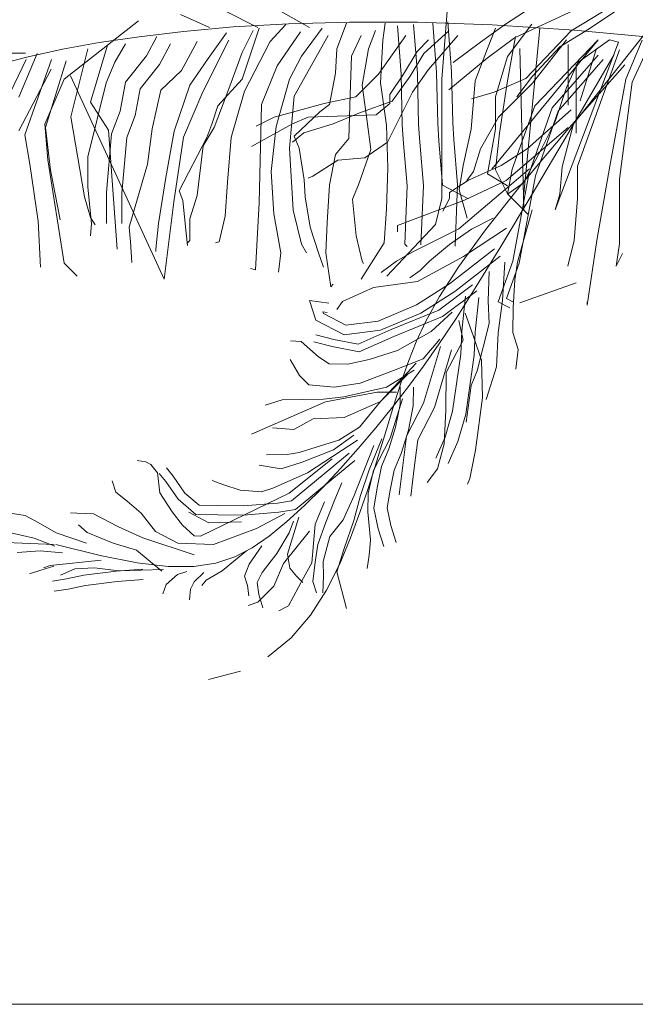
# Model space of a CAD drawing. Units: millimetres. Extents: x 595116 to 630915, y 909473 to 920225.
# Tile 96 of 134: x 629798.32 to 629805.27, y 919160.92 to 919172.02. Entities that reach past the tile are written whole.
import ezdxf

# ---------------------------------------------------------------- set-up
doc = ezdxf.new("R2010")
doc.units = ezdxf.units.MM
doc.layers.add('L-PLNT', color=85, linetype='Continuous', lineweight=13)

# ---------------------------------------------------------------- blocks, each defined once
blk = doc.blocks.new('A$C4FB75ABC')
for p, q in [((2.1065, 2.3741), (2.087, 2.1315)), ((2.2781, 2.2963), (2.353, 2.344)), ((2.3054, 2.2555), (2.4825, 2.3372)), ((2.5983, 2.3508), (2.4757, 2.2759)), ((2.6119, 2.3372), (2.5302, 2.2827)), ((1.3881, 2.2867), (1.3008, 2.3255)), ((1.5337, 2.2867), (1.4367, 2.3352)), ((1.6891, 2.2867), (1.6017, 2.3352)), ((1.1746, 2.3061), (0.9513, 2.1315)), ((1.4598, 2.2878), (1.3106, 2.2744)), ((1.6258, 2.2976), (1.4598, 2.2878)), ((1.5376, 2.2844), (1.4866, 2.1313)), ((1.6179, 2.2954), (1.5705, 2.2443)), ((1.8099, 2.3026), (1.6258, 2.2976)), ((1.7274, 2.2844), (1.6654, 2.2006)), ((1.8004, 2.299), (1.7712, 2.2224)), ((2.0136, 2.3019), (1.8099, 2.3026)), ((1.9171, 2.299), (1.9098, 2.248)), ((1.9536, 2.2917), (1.9646, 2.1459)), ((2.0023, 2.2954), (2.0134, 2.1483)), ((2.2382, 2.2942), (2.0136, 2.3019)), ((2.0597, 2.2997), (2.0708, 2.1511)), ((2.1047, 2.3031), (2.1159, 2.1533)), ((2.2032, 2.2419), (2.2781, 2.2963)), ((2.2482, 2.2839), (2.2239, 2.2232)), ((2.4852, 2.2785), (2.2382, 2.2942)), ((2.3575, 2.296), (2.2846, 2.199)), ((2.3818, 2.2839), (2.3332, 1.7863)), ((2.5302, 2.2827), (2.4416, 2.2282)), ((2.7559, 2.2536), (2.4852, 2.2785)), ((1.1767, 2.2586), (1.0564, 2.241)), ((1.3106, 2.2744), (1.1767, 2.2586)), ((1.23, 2.2589), (1.1992, 2.2008)), ((1.4391, 2.2699), (1.3844, 2.1933)), ((1.5194, 2.2771), (1.4866, 2.2115)), ((1.6617, 2.2735), (1.5924, 2.1714)), ((1.7456, 2.2626), (1.6435, 2.0802)), ((1.8442, 2.2626), (1.815, 2.2006)), ((1.8879, 2.2771), (1.8661, 2.2224)), ((1.9783, 2.2623), (1.8966, 2.1465)), ((2.0124, 2.2146), (2.0465, 2.2487)), ((2.1078, 2.2759), (2.0328, 2.2078)), ((2.135, 2.2623), (2.0465, 2.1602)), ((2.2236, 2.1942), (2.3054, 2.2555)), ((2.5574, 2.2487), (2.2372, 1.8605)), ((2.3089, 2.2596), (2.2846, 2.1261)), ((2.4757, 2.2759), (2.3394, 2.1329)), ((2.462, 2.2487), (2.3599, 2.1193)), ((2.3667, 2.0512), (2.5574, 2.2487)), ((2.6937, 2.2623), (2.4825, 1.9967)), ((2.5915, 2.2487), (2.4961, 2.1806)), ((2.6187, 2.2419), (2.5915, 2.2487)), ((0.9464, 2.2213), (0.8429, 2.1986)), ((1.0564, 2.241), (0.9464, 2.2213)), ((1.0231, 2.2224), (0.972, 2.0182)), ((1.0815, 2.2334), (1.0304, 2.062)), ((1.1363, 2.237), (1.1034, 2.1823)), ((1.2713, 2.237), (1.2384, 2.175)), ((1.3515, 2.2443), (1.3041, 2.1568)), ((1.4464, 2.2479), (1.3687, 2.0927)), ((1.5705, 2.2443), (1.4939, 2.0948)), ((1.7712, 2.2224), (1.7675, 2.1495)), ((1.8661, 2.2224), (1.8478, 2.113)), ((1.9098, 2.248), (1.9025, 2.1203)), ((2.1214, 2.1806), (2.2032, 2.2419)), ((2.2239, 2.2232), (2.1875, 2.1261)), ((2.3211, 2.2232), (2.3332, 1.7378)), ((2.4416, 2.2282), (2.3599, 2.1397)), ((2.428, 1.738), (2.6187, 2.2419)), ((2.4668, 2.2354), (2.4668, 2.0533)), ((2.6209, 2.2188), (2.4948, 1.8695)), ((2.5518, 2.2232), (2.5032, 2.0655)), ((2.6889, 2.2479), (2.6404, 2.1315)), ((2.7083, 2.2285), (2.6598, 2.1218)), ((0.837, 2.1896), (0.7276, 1.9635)), ((0.8429, 2.1986), (0.7422, 2.1723)), ((0.8348, 2.2091), (0.7572, 2.2091)), ((0.8699, 2.2079), (0.8151, 2.0766)), ((0.9137, 2.1896), (0.8334, 1.9635)), ((1.1992, 2.2008), (1.1362, 2.1221)), ((1.3844, 2.1933), (1.3297, 2.113)), ((1.4866, 2.2115), (1.4464, 2.1021)), ((1.6654, 2.2006), (1.6289, 2.1313)), ((1.815, 2.2006), (1.8113, 2.0838)), ((1.9715, 2.1465), (2.0124, 2.2146)), ((2.0328, 2.2078), (1.992, 2.1397)), ((2.1078, 2.0989), (2.2236, 2.1942)), ((2.2846, 2.199), (2.2482, 2.0776)), ((2.5572, 2.203), (2.4187, 2.0449)), ((2.5724, 2.1897), (2.4365, 2.0345)), ((2.6056, 2.2048), (2.4676, 1.9701)), ((0.9125, 2.1606), (0.8154, 1.9763)), ((0.9575, 2.186), (0.8954, 1.9854)), ((1.1034, 2.1823), (1.0779, 2.1203)), ((1.2384, 2.175), (1.18, 2.1021)), ((1.5924, 2.1714), (1.5449, 2.0547)), ((2.0465, 2.1602), (1.9988, 2.0921)), ((2.4961, 2.1806), (2.462, 2.1057)), ((2.6368, 2.1742), (2.4628, 1.9766)), ((2.4911, 2.1747), (2.4911, 1.9684)), ((0.9513, 2.1315), (0.8931, 1.9957)), ((1.2522, 1.53), (0.9707, 2.1412)), ((1.3041, 2.1568), (1.2421, 2.0984)), ((1.4866, 2.1313), (1.4136, 2.051)), ((1.6289, 2.1313), (1.5887, 1.989)), ((1.7675, 2.1495), (1.7493, 2.0547)), ((1.8966, 2.1465), (1.8285, 2.0784)), ((1.9306, 2.0852), (1.9715, 2.1465)), ((1.992, 2.1397), (1.9375, 2.0648)), ((1.9646, 2.1459), (1.9682, 1.9927)), ((2.0134, 2.1483), (2.017, 1.9949)), ((2.0708, 2.1511), (2.0745, 1.9975)), ((2.087, 2.1315), (2.087, 1.7725)), ((2.1159, 2.1533), (2.1196, 1.9995)), ((2.3394, 2.1329), (2.244, 2.0921)), ((2.3599, 2.1397), (2.3122, 2.0784)), ((2.6404, 2.1315), (2.5918, 1.8695)), ((1.0779, 2.1203), (1.0231, 1.8978)), ((1.1362, 2.1221), (1.1203, 2.0346)), ((1.18, 2.1021), (1.1654, 2.0218)), ((1.3297, 2.113), (1.2822, 1.9744)), ((1.4464, 2.1021), (1.4026, 1.9854)), ((1.8478, 2.113), (1.8624, 2.0036)), ((1.9025, 2.1203), (1.9208, 1.9927)), ((2.1875, 2.1261), (2.1754, 1.9805)), ((2.3599, 2.1193), (2.2577, 2.0172)), ((2.2846, 2.1261), (2.2604, 1.9684)), ((2.462, 2.1057), (2.428, 2.0035)), ((2.6598, 2.1218), (2.6209, 1.8307)), ((1.2421, 2.0984), (1.2165, 1.9817)), ((1.3687, 2.0927), (1.3105, 1.9569)), ((1.4939, 2.0948), (1.4537, 1.9562)), ((1.6435, 2.0802), (1.6289, 1.9234)), ((1.8285, 2.0784), (1.7331, 2.058)), ((1.8113, 2.0838), (1.8077, 1.9526)), ((1.9988, 2.0921), (1.9238, 1.9422)), ((1.9306, 2.058), (1.9306, 2.0852)), ((2.244, 2.0921), (2.1759, 2.0716)), ((2.2482, 2.0776), (2.2482, 1.9805)), ((1.0304, 2.062), (1.0852, 1.9781)), ((1.4136, 2.051), (1.3953, 1.9963)), ((1.5449, 2.0547), (1.5376, 1.7593)), ((1.7331, 2.058), (1.5832, 2.0172)), ((1.7493, 2.0547), (1.7201, 2.0328)), ((1.9375, 2.0648), (1.8421, 2.0308)), ((1.8898, 2.024), (1.9306, 2.058)), ((2.2985, 1.8605), (2.3667, 2.0512)), ((2.4187, 2.0449), (2.3489, 1.8456)), ((0.972, 2.0182), (1.0122, 1.7775)), ((1.1203, 2.0346), (1.0939, 1.9669)), ((1.1654, 2.0218), (1.1399, 1.9562)), ((1.5832, 2.0172), (1.5287, 1.9899)), ((1.6377, 1.9967), (1.6854, 2.0172)), ((1.7201, 2.0328), (1.6435, 1.9598)), ((1.6854, 2.0172), (1.8898, 2.024)), ((1.8421, 2.0308), (1.7603, 1.9967)), ((2.2577, 2.0172), (2.2032, 1.9218)), ((2.4756, 2.0387), (2.3438, 1.9217)), ((2.4365, 2.0345), (2.3686, 1.8404)), ((0.8931, 1.9957), (0.9028, 1.8889)), ((0.8954, 1.9854), (0.91, 1.8577)), ((1.4026, 1.9854), (1.3698, 1.9307)), ((1.3953, 1.9963), (1.3807, 1.9562)), ((1.5151, 1.9286), (1.6377, 1.9967)), ((1.5887, 1.989), (1.5741, 1.8541)), ((1.7603, 1.9967), (1.6718, 1.9695)), ((1.8624, 2.0036), (1.8734, 1.9197)), ((1.9208, 1.9927), (1.9244, 1.865)), ((1.9682, 1.9927), (1.9719, 1.938)), ((2.017, 1.9949), (2.0206, 1.9417)), ((2.0745, 1.9975), (2.0779, 1.946)), ((2.1196, 1.9995), (2.1229, 1.9495)), ((2.4673, 1.986), (2.2802, 1.8264)), ((2.428, 2.0035), (2.3871, 1.9218)), ((2.4825, 1.9967), (2.4484, 1.8673)), ((0.8334, 1.9635), (0.848, 1.876)), ((1.0939, 1.9669), (1.0786, 1.7905)), ((1.0852, 1.9781), (1.1107, 1.6207)), ((1.1399, 1.9562), (1.1253, 1.7884)), ((1.2165, 1.9817), (1.2019, 1.876)), ((1.2822, 1.9744), (1.2567, 1.8358)), ((1.3105, 1.9569), (1.2814, 1.7628)), ((1.3807, 1.9562), (1.2968, 1.7957)), ((1.4537, 1.9562), (1.4428, 1.8213)), ((1.6718, 1.9695), (1.6377, 1.9422)), ((1.6435, 1.9598), (1.6581, 1.9234)), ((1.8077, 1.9526), (1.7675, 1.9051)), ((2.1754, 1.9805), (2.1511, 1.8713)), ((2.2482, 1.9805), (2.2239, 1.847)), ((2.2604, 1.9684), (2.2482, 1.8591)), ((2.4628, 1.9766), (2.3249, 1.8127)), ((2.4676, 1.9701), (2.3552, 1.7802)), ((1.3698, 1.9307), (1.3515, 1.7811)), ((1.6289, 1.9234), (1.6398, 1.7374)), ((1.6581, 1.9234), (1.6727, 1.8285)), ((1.9238, 1.9422), (1.8557, 1.8946)), ((1.9719, 1.938), (1.9828, 1.8103)), ((2.0206, 1.9417), (2.0317, 1.8114)), ((2.0779, 1.946), (2.0893, 1.8127)), ((2.1229, 1.9495), (2.1345, 1.8136)), ((1.0231, 1.8978), (1.0231, 1.8067)), ((1.7675, 1.9051), (1.7493, 1.814)), ((1.8557, 1.8946), (1.7739, 1.8878)), ((1.8734, 1.9197), (1.8369, 1.814)), ((2.2032, 1.9218), (2.1827, 1.8537)), ((2.3438, 1.9217), (2.2657, 1.8718)), ((2.3871, 1.9218), (2.3326, 1.8197)), ((0.848, 1.876), (0.8735, 1.7045)), ((0.9028, 1.8889), (0.9513, 1.5785)), ((1.2019, 1.876), (1.1472, 1.6863)), ((1.7739, 1.8878), (1.699, 1.8401)), ((1.9244, 1.865), (1.9208, 1.741)), ((2.1511, 1.8713), (2.1389, 1.7985)), ((2.2657, 1.8718), (2.167, 1.8279)), ((2.4484, 1.8673), (2.4416, 1.7856)), ((2.4948, 1.8695), (2.4948, 1.7725)), ((2.5918, 1.8695), (2.553, 1.6464)), ((0.91, 1.8577), (0.9392, 1.7082)), ((1.2567, 1.8358), (1.2348, 1.6973)), ((1.5741, 1.8541), (1.5814, 1.7264)), ((1.699, 1.8401), (1.6854, 1.8333)), ((2.3505, 1.8613), (2.1386, 1.6813)), ((2.1827, 1.8537), (2.1623, 1.8265)), ((2.2239, 1.847), (2.2846, 1.8106)), ((2.2482, 1.8591), (2.2846, 1.7863)), ((2.2849, 1.7856), (2.2985, 1.8605)), ((2.3489, 1.8456), (2.3004, 1.5838)), ((2.3686, 1.8404), (2.32, 1.5785)), ((1.0231, 1.8067), (1.0341, 1.6973)), ((1.4428, 1.8213), (1.4355, 1.7191)), ((1.6727, 1.8285), (1.6763, 1.7775)), ((1.7493, 1.814), (1.742, 1.7009)), ((1.8369, 1.814), (1.8186, 1.7702)), ((1.9828, 1.8103), (1.9755, 1.6352)), ((2.0317, 1.8114), (2.0243, 1.6332)), ((2.0893, 1.8127), (2.1647, 1.7725)), ((2.167, 1.8279), (2.1099, 1.791)), ((2.1345, 1.8136), (2.1268, 1.6289)), ((2.2802, 1.8264), (2.1549, 1.7678)), ((2.3249, 1.8127), (2.2184, 1.678)), ((2.3326, 1.8197), (2.2849, 1.7856)), ((2.6209, 1.8307), (2.6209, 1.6367)), ((1.0122, 1.7775), (1.0304, 1.7155)), ((1.0786, 1.7905), (1.0786, 1.6973)), ((1.1253, 1.7884), (1.1253, 1.7665)), ((1.2968, 1.7957), (1.3078, 1.7665)), ((1.3515, 1.7811), (1.3297, 1.7118)), ((1.6763, 1.7775), (1.6909, 1.6863)), ((2.1099, 1.791), (2.1096, 1.7722)), ((2.1389, 1.7985), (2.1632, 1.7135)), ((2.3552, 1.7802), (2.2641, 1.6283)), ((2.2846, 1.7863), (2.3453, 1.7256)), ((2.4416, 1.7856), (2.428, 1.738)), ((1.1253, 1.7665), (1.1253, 1.7301)), ((1.2814, 1.7628), (1.2522, 1.53)), ((1.3078, 1.7665), (1.3187, 1.6681)), ((1.5376, 1.7593), (1.5267, 1.5587)), ((1.8186, 1.7702), (1.8296, 1.6608)), ((2.1549, 1.7678), (1.9538, 1.6913)), ((2.087, 1.7725), (2.0676, 1.6949)), ((2.1096, 1.7722), (2.0903, 1.7347)), ((2.4948, 1.7725), (2.485, 1.6464)), ((1.1253, 1.7301), (1.1253, 1.6973)), ((1.4355, 1.7191), (1.4172, 1.6425)), ((1.5814, 1.7264), (1.6033, 1.6097)), ((1.6398, 1.7374), (1.6654, 1.6352)), ((1.9208, 1.741), (1.9135, 1.6389)), ((2.3582, 1.7386), (2.3145, 1.5808)), ((0.8735, 1.7045), (0.8808, 1.566)), ((1.0304, 1.7155), (1.045, 1.6936)), ((1.0341, 1.6973), (1.0304, 1.6608)), ((1.1472, 1.6863), (1.1509, 1.6425)), ((1.2348, 1.6973), (1.2275, 1.6207)), ((1.3297, 1.7118), (1.3297, 1.6462)), ((1.6909, 1.6863), (1.7164, 1.6097)), ((1.742, 1.7009), (1.7383, 1.6097)), ((2.0676, 1.6949), (1.922, 1.5397)), ((1.9538, 1.6913), (1.9536, 1.6725)), ((2.2409, 1.7138), (2.1763, 1.6807)), ((1.3187, 1.6681), (1.3224, 1.6316)), ((1.8296, 1.6608), (1.8478, 1.5842)), ((2.1386, 1.6813), (1.998, 1.6115)), ((2.1763, 1.6807), (2.1096, 1.6345)), ((2.2184, 1.678), (2.1385, 1.568)), ((2.2819, 1.6831), (2.1525, 1.5981)), ((1.1509, 1.6425), (1.1545, 1.5805)), ((1.3297, 1.6462), (1.3224, 1.6389)), ((1.4172, 1.6425), (1.4063, 1.6389)), ((1.6654, 1.6352), (1.68, 1.6097)), ((1.9135, 1.6389), (1.8444, 1.53)), ((1.9755, 1.6352), (1.9828, 1.628)), ((2.1096, 1.6345), (2.0504, 1.5844)), ((2.2641, 1.6283), (2.1904, 1.5079)), ((2.485, 1.6464), (2.4656, 1.5688)), ((2.553, 1.6464), (2.5239, 1.4523)), ((2.6209, 1.6367), (2.6112, 1.5688)), ((1.2275, 1.6207), (1.2275, 1.6134)), ((1.6033, 1.6097), (1.596, 1.5514)), ((1.7164, 1.6097), (1.731, 1.566)), ((1.7383, 1.6097), (1.7529, 1.5076)), ((1.998, 1.6115), (1.9504, 1.5839)), ((2.1525, 1.5981), (2.0137, 1.5227)), ((2.2452, 1.6213), (2.1098, 1.5157)), ((2.2623, 1.5995), (2.1258, 1.493)), ((2.6112, 1.5688), (2.6307, 1.6076)), ((0.9513, 1.5785), (0.9901, 1.5397)), ((1.8478, 1.5842), (1.8515, 1.5769)), ((1.9504, 1.5839), (1.9047, 1.5506)), ((2.0504, 1.5844), (2.0217, 1.5565)), ((2.1385, 1.568), (2.0803, 1.4783)), ((2.3004, 1.5838), (2.256, 1.4617)), ((2.2767, 1.5813), (2.2695, 1.4664)), ((2.32, 1.5785), (2.2812, 1.4717)), ((2.3145, 1.5808), (2.3062, 1.5281)), ((1.5267, 1.5587), (1.5121, 1.5623)), ((2.0217, 1.5565), (1.9912, 1.5343)), ((2.2292, 1.5537), (2.2261, 1.4651)), ((1.7529, 1.5076), (1.7602, 1.5149)), ((2.0137, 1.5227), (1.8814, 1.5056)), ((2.1098, 1.5157), (2.0109, 1.453)), ((2.1796, 1.5129), (2.0785, 1.437)), ((2.3062, 1.5281), (2.3013, 1.4452)), ((2.4911, 1.5193), (2.3211, 1.4586)), ((1.8814, 1.5056), (1.7884, 1.4636)), ((2.1258, 1.493), (2.0238, 1.4284)), ((2.1927, 1.4954), (2.0894, 1.4177)), ((2.1904, 1.5079), (2.1298, 1.4122)), ((2.1578, 1.4791), (2.1468, 1.3743)), ((1.7084, 1.4073), (1.6895, 1.4666)), ((1.6895, 1.4666), (1.747, 1.4576)), ((1.7884, 1.4636), (1.7711, 1.4393)), ((2.0109, 1.453), (1.8951, 1.4036)), ((2.0803, 1.4783), (2.039, 1.4043)), ((2.1979, 1.4749), (2.187, 1.3714)), ((2.2261, 1.4651), (2.2289, 1.3972)), ((2.256, 1.4617), (2.2916, 1.4439)), ((2.2695, 1.4664), (2.2568, 1.3685)), ((2.2812, 1.4717), (2.3006, 1.462)), ((2.5239, 1.4523), (2.5239, 1.462)), ((1.7313, 1.4266), (1.7295, 1.4323)), ((1.7295, 1.4323), (1.7427, 1.4302)), ((1.7987, 1.3918), (1.7313, 1.4266)), ((2.0238, 1.4284), (1.9024, 1.3766)), ((2.0785, 1.437), (1.9344, 1.3786)), ((2.1181, 1.4308), (2.055, 1.3732)), ((2.1569, 1.4277), (2.1816, 1.3609)), ((2.3013, 1.4452), (2.3002, 1.3698)), ((1.7936, 1.3632), (1.7084, 1.4073)), ((1.8951, 1.4036), (1.7987, 1.3918)), ((2.0894, 1.4177), (1.9429, 1.3584)), ((2.039, 1.4043), (2.0098, 1.3416)), ((2.1298, 1.4122), (2.0784, 1.3347)), ((2.1385, 1.406), (2.1509, 1.3473)), ((2.2289, 1.3972), (2.1929, 1.2544)), ((1.7623, 1.3489), (1.7078, 1.3628)), ((1.9024, 1.3766), (1.7936, 1.3632)), ((1.9344, 1.3786), (1.8357, 1.3347)), ((2.055, 1.3732), (1.9542, 1.3161)), ((2.1468, 1.3743), (2.1439, 1.3053)), ((2.1816, 1.3609), (2.2062, 1.287)), ((2.187, 1.3714), (2.1842, 1.3016)), ((2.2568, 1.3685), (2.2516, 1.2668)), ((2.3002, 1.3698), (2.3165, 1.3187)), ((1.6641, 1.3427), (1.6321, 1.345)), ((1.7163, 1.2967), (1.6641, 1.3427)), ((1.7575, 1.3275), (1.7024, 1.3416)), ((1.8357, 1.3347), (1.7623, 1.3489)), ((1.9429, 1.3584), (1.8383, 1.3119)), ((2.0098, 1.3416), (1.9878, 1.2857)), ((2.0811, 1.3502), (2.0312, 1.2905)), ((2.0784, 1.3347), (2.0319, 1.2687)), ((2.1509, 1.3473), (2.1005, 1.25)), ((1.8383, 1.3119), (1.7575, 1.3275)), ((1.9542, 1.3161), (1.869, 1.289)), ((2.0829, 1.3276), (2.0324, 1.158)), ((2.1165, 1.3176), (2.065, 1.1449)), ((2.1439, 1.3053), (2.1195, 1.1332)), ((2.1842, 1.3016), (2.1591, 1.1247)), ((2.3165, 1.3187), (2.31, 1.2603)), ((1.6589, 1.2409), (1.6313, 1.2885)), ((1.7481, 1.2755), (1.7163, 1.2967)), ((1.8046, 1.2748), (1.7481, 1.2755)), ((1.869, 1.289), (1.8046, 1.2748)), ((2.0103, 1.2776), (1.903, 1.1622)), ((2.0312, 1.2905), (1.9421, 1.2559)), ((1.9878, 1.2857), (1.9691, 1.2327)), ((2.2062, 1.287), (2.2097, 1.1745)), ((1.9421, 1.2559), (1.8416, 1.2177)), ((1.9834, 1.244), (1.903, 1.1622)), ((2.0043, 1.257), (1.9206, 1.2053)), ((2.0319, 1.2687), (1.9864, 1.2075)), ((2.1005, 1.25), (2.0989, 1.1369)), ((2.1929, 1.2544), (2.1754, 1.2112)), ((2.2516, 1.2668), (2.22, 1.1691)), ((1.6868, 1.2123), (1.6589, 1.2409)), ((1.8416, 1.2177), (1.7641, 1.2056)), ((1.9691, 1.2327), (1.952, 1.1808)), ((1.7641, 1.2056), (1.6868, 1.2123)), ((1.7376, 1.1613), (1.8929, 1.1904)), ((1.9206, 1.2053), (1.792, 1.1769)), ((1.8929, 1.1904), (1.9511, 1.1904)), ((1.9864, 1.2075), (1.9386, 1.1458)), ((1.9621, 1.2066), (1.9614, 1.1536)), ((2.0017, 1.2061), (2.001, 1.1495)), ((2.1754, 1.2112), (2.1606, 1.1002)), ((1.5143, 1.0642), (1.7376, 1.1613)), ((1.607, 1.1681), (1.5558, 1.1518)), ((1.7315, 1.1702), (1.607, 1.1681)), ((1.792, 1.1769), (1.7315, 1.1702)), ((1.903, 1.1622), (1.793, 1.1147)), ((1.903, 1.1622), (1.8397, 1.0857)), ((1.9692, 1.1707), (1.9317, 1.0524)), ((1.952, 1.1808), (1.9358, 1.129)), ((1.9614, 1.1536), (1.9482, 1.0859)), ((2.0324, 1.158), (1.9806, 1.0581)), ((2.2097, 1.1745), (2.1886, 1.0162)), ((1.9386, 1.1458), (1.8882, 1.0835)), ((1.9358, 1.129), (1.9198, 1.076)), ((2.001, 1.1495), (1.9867, 1.0762)), ((2.065, 1.1449), (2.0146, 1.0475)), ((2.0989, 1.1369), (2.0937, 1.0351)), ((2.1195, 1.1332), (2.0972, 1.056)), ((2.1591, 1.1247), (2.1353, 1.0421)), ((1.7005, 1.1103), (1.6416, 1.079)), ((1.793, 1.1147), (1.7005, 1.1103)), ((1.6416, 1.079), (1.5775, 1.0837)), ((1.8397, 1.0857), (1.7769, 1.047)), ((1.8882, 1.0835), (1.8359, 1.0215)), ((1.9198, 1.076), (1.903, 1.0206)), ((1.9482, 1.0859), (1.9278, 1.0204)), ((1.9867, 1.0762), (1.965, 1.0067)), ((1.8335, 1.0462), (1.6831, 0.9483)), ((1.7769, 1.047), (1.7087, 1.0253)), ((1.8224, 1.0615), (1.7614, 1.017)), ((1.9071, 1.0509), (1.8681, 0.9571)), ((1.9317, 1.0524), (1.8813, 0.9551)), ((1.9806, 1.0581), (1.9586, 0.8825)), ((2.0146, 1.0475), (2.004, 0.9628)), ((2.0972, 1.056), (2.0692, 0.9929)), ((2.1353, 1.0421), (2.1061, 0.9765)), ((1.6576, 1.009), (1.6216, 1.0039)), ((1.8084, 1.007), (1.6348, 0.8642)), ((1.7087, 1.0253), (1.6576, 1.009)), ((1.7614, 1.017), (1.6666, 0.9806)), ((1.8359, 1.0215), (1.7823, 0.9612)), ((1.8823, 1.0305), (1.8549, 0.9592)), ((1.903, 1.0206), (1.8847, 0.9618)), ((1.9278, 1.0204), (1.9055, 0.9679)), ((1.965, 1.0067), (1.9435, 0.9561)), ((2.0937, 1.0351), (2.0738, 0.96)), ((2.1886, 1.0162), (2.171, 0.9318)), ((1.1969, 0.9814), (1.1705, 0.9855)), ((1.2119, 0.9737), (1.1969, 0.9814)), ((1.6216, 1.0039), (1.5594, 1.0028)), ((1.6666, 0.9806), (1.6041, 0.9607)), ((1.7573, 0.9907), (1.6276, 0.8869)), ((1.8259, 0.9857), (1.6466, 0.8382)), ((1.2323, 0.9489), (1.2119, 0.9737)), ((1.239, 0.8884), (1.2323, 0.9489)), ((1.2793, 0.9388), (1.2589, 0.9636)), ((1.6041, 0.9607), (1.5382, 0.9711)), ((1.6831, 0.9483), (1.5787, 0.9026)), ((1.7823, 0.9612), (1.7281, 0.9036)), ((1.8549, 0.9592), (1.8236, 0.8804)), ((1.8681, 0.9571), (1.8425, 0.8802)), ((1.8847, 0.9618), (1.8642, 0.8983)), ((1.8813, 0.9551), (1.8652, 0.8874)), ((1.9055, 0.9679), (1.8924, 0.9029)), ((1.9435, 0.9561), (1.9314, 0.8959)), ((2.004, 0.9628), (1.9934, 0.8781)), ((2.0738, 0.96), (2.043, 0.9189)), ((1.107, 0.8902), (1.0961, 0.9243)), ((1.2572, 0.9222), (1.2376, 0.9461)), ((1.2938, 0.8688), (1.2572, 0.9222)), ((1.3144, 0.8874), (1.2793, 0.9388)), ((1.4036, 0.922), (1.3961, 0.9259)), ((1.4317, 0.9122), (1.4036, 0.922)), ((1.7864, 0.9186), (1.765, 0.868)), ((2.171, 0.9318), (2.164, 0.9142)), ((1.1405, 0.8634), (1.107, 0.8902)), ((1.2759, 0.8314), (1.239, 0.8884)), ((1.3573, 0.851), (1.3144, 0.8874)), ((1.4805, 0.8964), (1.4317, 0.9122)), ((1.5446, 0.8918), (1.4805, 0.8964)), ((1.5787, 0.9026), (1.5446, 0.8918)), ((1.7281, 0.9036), (1.6739, 0.8498)), ((1.8642, 0.8983), (1.8405, 0.829)), ((1.8652, 0.8874), (1.8644, 0.8308)), ((1.8924, 0.9029), (1.8829, 0.8424)), ((1.9314, 0.8959), (1.9231, 0.8432)), ((1.1834, 0.827), (1.1405, 0.8634)), ((1.347, 0.8236), (1.2938, 0.8688)), ((1.6276, 0.8869), (1.3617, 0.7585)), ((1.6348, 0.8642), (1.5932, 0.8572)), ((1.7347, 0.8614), (1.7065, 0.7946)), ((1.765, 0.868), (1.7376, 0.7967)), ((1.8236, 0.8804), (1.7906, 0.8073)), ((1.8425, 0.8802), (1.8226, 0.805)), ((1.3074, 0.7913), (1.2759, 0.8314)), ((1.3863, 0.7981), (1.3265, 0.8298)), ((1.4139, 0.8502), (1.3573, 0.851)), ((1.4893, 0.8492), (1.4139, 0.8502)), ((1.5932, 0.8572), (1.4893, 0.8492)), ((1.5965, 0.8298), (1.4902, 0.8216)), ((1.6466, 0.8382), (1.5965, 0.8298)), ((1.6739, 0.8498), (1.6204, 0.8011)), ((1.8405, 0.829), (1.8129, 0.7535)), ((1.8644, 0.8308), (1.8727, 0.7459)), ((1.8829, 0.8424), (1.8952, 0.7804)), ((1.9231, 0.8432), (1.9337, 0.7903)), ((0.8346, 0.8198), (0.7888, 0.827)), ((0.8736, 0.7996), (0.8346, 0.8198)), ((0.9273, 0.7678), (0.8736, 0.7996)), ((0.9891, 0.8277), (0.9703, 0.828)), ((1.04, 0.8252), (0.9891, 0.8277)), ((1.1149, 0.7864), (1.04, 0.8252)), ((1.226, 0.7717), (1.1834, 0.827)), ((1.4135, 0.8227), (1.347, 0.8236)), ((1.4848, 0.8016), (1.3863, 0.7981)), ((1.4902, 0.8216), (1.4135, 0.8227)), ((1.6154, 0.8267), (1.5299, 0.7807)), ((1.6204, 0.8011), (1.5682, 0.7585)), ((1.6567, 0.8148), (1.6231, 0.704)), ((1.6415, 0.8037), (1.6278, 0.7681)), ((1.7906, 0.8073), (1.7502, 0.757)), ((1.8226, 0.805), (1.7931, 0.7206)), ((1.0204, 0.7689), (0.9943, 0.7918)), ((1.188, 0.7534), (1.1149, 0.7864)), ((1.2935, 0.7368), (1.226, 0.7717)), ((1.3428, 0.7588), (1.3074, 0.7913)), ((1.5299, 0.7807), (1.4009, 0.7335)), ((1.6891, 0.7732), (1.6114, 0.6762)), ((1.7065, 0.7946), (1.696, 0.6785)), ((1.7376, 0.7967), (1.7141, 0.733)), ((1.8952, 0.7804), (1.9122, 0.7271)), ((1.9337, 0.7903), (1.9499, 0.7392)), ((0.9219, 0.7334), (0.7236, 0.7411)), ((0.8615, 0.7523), (0.7912, 0.768)), ((0.9235, 0.7285), (0.8615, 0.7523)), ((1.0187, 0.737), (0.9273, 0.7678)), ((1.0992, 0.7376), (1.0204, 0.7689)), ((1.342, 0.7022), (1.188, 0.7534)), ((1.3617, 0.7585), (1.3428, 0.7588)), ((1.5682, 0.7585), (1.5172, 0.7231)), ((1.6278, 0.7681), (1.5911, 0.7064)), ((1.7502, 0.757), (1.7303, 0.6818)), ((1.8129, 0.7535), (1.7799, 0.6746)), ((1.8727, 0.7459), (1.8683, 0.7007)), ((0.879, 0.7143), (0.8101, 0.7087)), ((0.9462, 0.7085), (0.879, 0.7143)), ((1.0599, 0.6997), (0.9265, 0.7333)), ((1.1687, 0.7159), (1.0992, 0.7376)), ((1.2451, 0.6526), (1.1687, 0.7159)), ((1.4009, 0.7335), (1.2935, 0.7368)), ((1.5006, 0.7151), (1.4262, 0.6539)), ((1.5172, 0.7231), (1.4647, 0.6957)), ((1.5461, 0.7296), (1.5076, 0.6736)), ((1.7141, 0.733), (1.7058, 0.6803)), ((1.7931, 0.7206), (1.7714, 0.6511)), ((1.0623, 0.6856), (0.9095, 0.6697)), ((1.1712, 0.6779), (1.0599, 0.6997)), ((1.4647, 0.6957), (1.4072, 0.6768)), ((1.5911, 0.7064), (1.5469, 0.6485)), ((1.6231, 0.704), (1.6301, 0.6625)), ((1.7303, 0.6818), (1.7316, 0.6384)), ((1.8683, 0.7007), (1.8621, 0.6612)), ((0.8811, 0.6557), (0.847, 0.6449)), ((0.9209, 0.6684), (0.8811, 0.6557)), ((0.9095, 0.6697), (0.8898, 0.6634)), ((0.9832, 0.6605), (0.9403, 0.6414)), ((1.0423, 0.6629), (0.9832, 0.6605)), ((1.1074, 0.6526), (1.011, 0.6408)), ((1.1159, 0.6537), (1.0423, 0.6629)), ((1.1867, 0.6591), (1.1074, 0.6526)), ((1.2504, 0.6584), (1.1159, 0.6537)), ((1.2639, 0.6673), (1.1712, 0.6779)), ((1.3414, 0.6671), (1.2639, 0.6673)), ((1.3206, 0.6516), (1.2921, 0.6426)), ((1.4072, 0.6768), (1.3414, 0.6671)), ((1.4262, 0.6539), (1.3787, 0.6263)), ((1.5076, 0.6736), (1.4939, 0.6379)), ((1.6114, 0.6762), (1.5823, 0.6082)), ((1.6301, 0.6625), (1.6505, 0.6377)), ((1.696, 0.6785), (1.6713, 0.6328)), ((1.7058, 0.6803), (1.6993, 0.6219)), ((1.7799, 0.6746), (1.74, 0.5958)), ((1.7714, 0.6511), (1.8, 0.5413)), ((0.9581, 0.6302), (0.9165, 0.6232)), ((1.011, 0.6408), (0.9581, 0.6302)), ((1.1106, 0.6216), (1.016, 0.61)), ((1.1893, 0.628), (1.1106, 0.6216)), ((1.2921, 0.6426), (1.2578, 0.6129)), ((1.3714, 0.649), (1.3428, 0.6211)), ((1.3787, 0.6263), (1.3652, 0.6095)), ((1.4939, 0.6379), (1.5029, 0.6095)), ((1.5469, 0.6485), (1.5314, 0.6186)), ((1.6713, 0.6328), (1.6256, 0.5484)), ((1.6505, 0.6377), (1.6691, 0.6186)), ((1.6993, 0.6219), (1.7101, 0.5878)), ((1.7316, 0.6384), (1.729, 0.5876)), ((0.9632, 0.5994), (0.9216, 0.5925)), ((1.016, 0.61), (0.9632, 0.5994)), ((1.2578, 0.6129), (1.2479, 0.5847)), ((1.3311, 0.5987), (1.3288, 0.5666)), ((1.3428, 0.6211), (1.3311, 0.5987)), ((1.5029, 0.6095), (1.5063, 0.5793)), ((1.5314, 0.6186), (1.5365, 0.5827)), ((1.5823, 0.6082), (1.5337, 0.5597)), ((1.74, 0.5958), (1.6917, 0.5207)), ((1.5365, 0.5827), (1.5492, 0.5429)), ((1.5337, 0.5597), (1.5046, 0.55)), ((1.6256, 0.5484), (1.5974, 0.5343)), ((1.6917, 0.5207), (1.6336, 0.4527)), ((1.6336, 0.4527), (1.5642, 0.3956)), ((1.4819, 0.3527), (1.3853, 0.3277))]:
    blk.add_line(p, q)

msp = doc.modelspace()

# ---------------------------------------------------------------- linework, layer by layer
at = {"layer": 'L-PLNT'}
msp.add_line((629511.274, 919160.917), (629824.951, 919160.917), dxfattribs=at)

# ---------------------------------------------------------------- block references
at = {"layer": 'L-PLNT', "xscale": 3.753413438031968, "yscale": 3.753413438031968, "zscale": 3.753413438031968}
msp.add_blockref('A$C4FB75ABC', (629795.248, 919163.35), dxfattribs=at)

doc.saveas('drawing.dxf')
